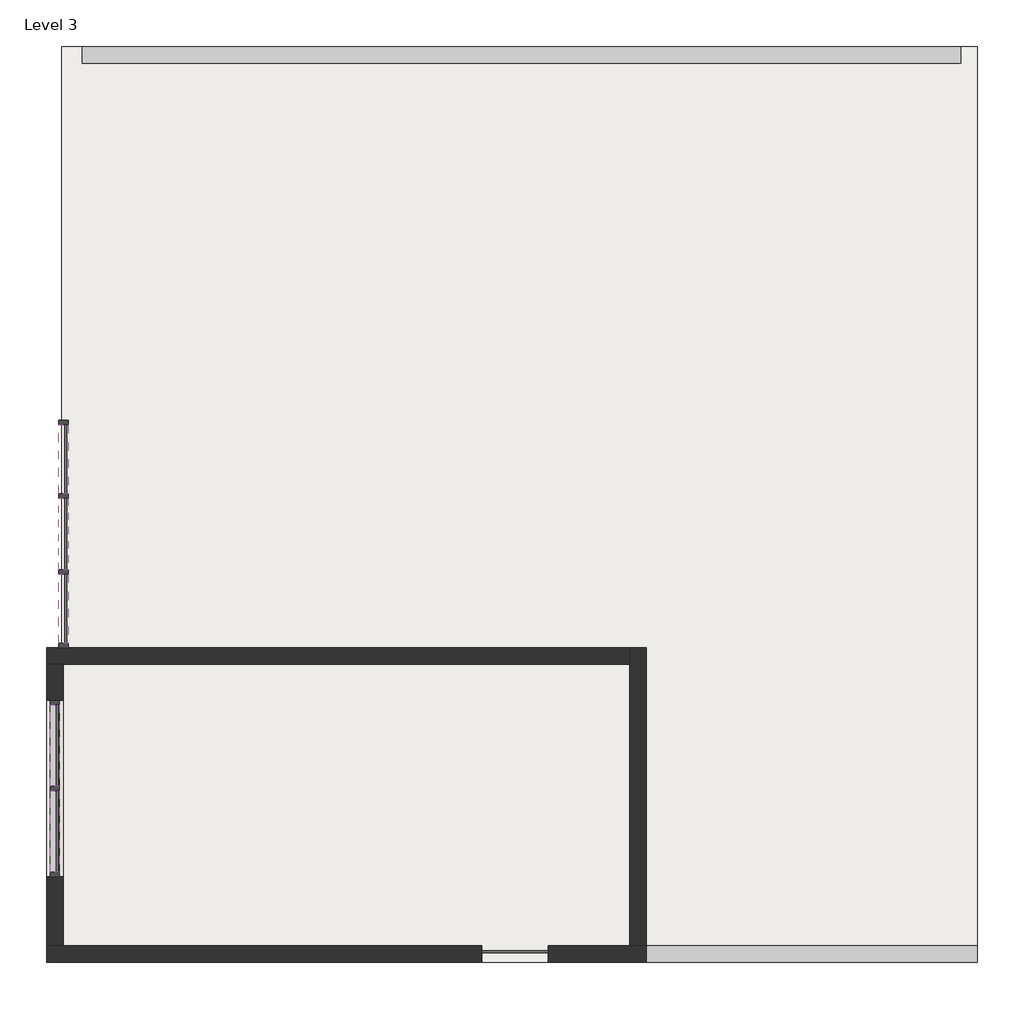
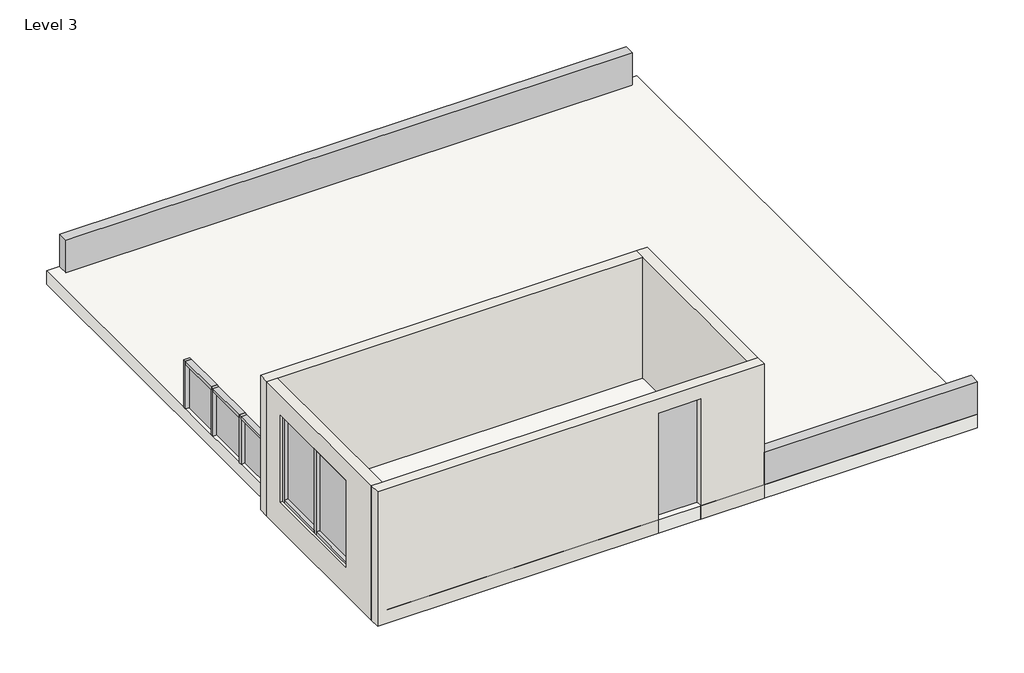
# One storey: 14 members, 7 plates, 4 walls, 2 proxies, 1 roof.
"""IFC4 building model written with IfcOpenShell, lengths in millimetres."""

from ifc_helpers import new_model, si_unit, frame, origin, place, context, project, spatial, polyline, outline, extrude, faceted_brep, transform, mapped, element, save
from components import generic_models_7_generic_models_7_f087c847, generic_models_9_generic_models_9_ac56366f, member_ade69111, member_05cf8435, member_3f9fbe84, member_9c6a9240, member_e6b9f524, member_bbdb212f, member_37619358, system_panel_glazed_77e7111d, system_panel_glazed_c8b910d9, system_panel_glazed_8012c4e8, system_panel_glazed_450ffc3c, system_panel_glazed_9aa1dd94

model = new_model("IFC4")

# Units and contexts
model_context = context("Model", 3, world=origin())
ifc_project = project(units=[si_unit("LENGTHUNIT", "METRE", prefix="MILLI")], contexts=[model_context])

# Site, building, storey
site = spatial("IfcSite", under=ifc_project)
building = spatial("IfcBuilding", under=site)
storey = spatial("IfcBuildingStorey", under=building, Name="Level 3", Elevation=6096.0)

# Proxies
placement = place(None, origin())
generic_models_7_generic_models_7_shape = generic_models_7_generic_models_7_f087c847(model_context)
element("IfcBuildingElementProxy", 1, Name="Generic Models 7 : Generic Models 7", ObjectType="Generic Models 7 : Generic Models 7", at=placement, inside=storey, context=model_context, shape_type="MappedRepresentation", body=[
    mapped(generic_models_7_generic_models_7_shape, transform((0.0, 0.0, 0.0), x_axis=(1.0, 0.0, 0.0), y_axis=(0.0, 1.0, 0.0), z_axis=(0.0, 0.0, 1.0))),
])
generic_models_9_generic_models_9_shape = generic_models_9_generic_models_9_ac56366f(model_context)
element("IfcBuildingElementProxy", 2, Name="Generic Models 9 : Generic Models 9", ObjectType="Generic Models 9 : Generic Models 9", at=placement, inside=storey, context=model_context, shape_type="MappedRepresentation", body=[
    mapped(generic_models_9_generic_models_9_shape, transform((0.0, 0.0, 0.0), x_axis=(1.0, 0.0, 0.0), y_axis=(0.0, 1.0, 0.0), z_axis=(0.0, 0.0, 1.0))),
])

# Members
member_shape = member_ade69111(model_context)
element("IfcMember", 3, ObjectType="Rectangular Mullion : 2.5\" x 5\" rectangular", at=placement, inside=storey, context=model_context, shape_type="MappedRepresentation", body=[
    mapped(member_shape, transform((-20241.3334471, -7434.170098, 6457.2827682), x_axis=(0.0, -1.0, 0.0), y_axis=(-1.0, 0.0, 0.0), z_axis=(0.0, 0.0, -1.0))),
])
element("IfcMember", 4, ObjectType="Rectangular Mullion : 2.5\" x 5\" rectangular", at=placement, inside=storey, context=model_context, shape_type="MappedRepresentation", body=[
    mapped(member_shape, transform((-20241.3334471, -8482.0613656, 6457.2827682), x_axis=(0.0, -1.0, 0.0), y_axis=(-1.0, 0.0, 0.0), z_axis=(0.0, 0.0, -1.0))),
])
member_2_shape = member_05cf8435(model_context)
element("IfcMember", 5, ObjectType="Rectangular Mullion : 2.5\" x 5\" rectangular", at=placement, inside=storey, context=model_context, shape_type="MappedRepresentation", body=[
    mapped(member_2_shape, transform((-20241.3334471, -8450.3113656, 7537.0329538), x_axis=(0.0, 0.0, 1.0), y_axis=(-1.0, 0.0, 0.0), z_axis=(0.0, -1.0, 0.0))),
])
member_3_shape = member_3f9fbe84(model_context)
element("IfcMember", 6, ObjectType="Rectangular Mullion : 2.5\" x 5\" rectangular", at=placement, inside=storey, context=model_context, shape_type="MappedRepresentation", body=[
    mapped(member_3_shape, transform((-20241.3334471, -7402.420098, 7537.0329538), x_axis=(0.0, 0.0, 1.0), y_axis=(-1.0, 0.0, 0.0), z_axis=(0.0, -1.0, 0.0))),
])
element("IfcMember", 7, ObjectType="Rectangular Mullion : 2.5\" x 5\" rectangular", at=placement, inside=storey, context=model_context, shape_type="MappedRepresentation", body=[
    mapped(member_3_shape, transform((-20241.3334471, -9466.4526331, 7537.0329538), x_axis=(0.0, 0.0, 1.0), y_axis=(-1.0, 0.0, 0.0), z_axis=(0.0, -1.0, 0.0))),
])
member_4_shape = member_9c6a9240(model_context)
element("IfcMember", 8, ObjectType="Rectangular Mullion : 2.5\" x 5\" rectangular", at=placement, inside=storey, context=model_context, shape_type="MappedRepresentation", body=[
    mapped(member_4_shape, transform((-20241.3334471, -6386.2788305, 7537.0329538), x_axis=(0.0, 1.0, 0.0), y_axis=(-1.0, 0.0, 0.0), z_axis=(0.0, 0.0, 1.0))),
])
element("IfcMember", 9, ObjectType="Rectangular Mullion : 2.5\" x 5\" rectangular", at=placement, inside=storey, context=model_context, shape_type="MappedRepresentation", body=[
    mapped(member_4_shape, transform((-20241.3334471, -9529.9526331, 6457.2827682), x_axis=(0.0, -1.0, 0.0), y_axis=(-1.0, 0.0, 0.0), z_axis=(0.0, 0.0, -1.0))),
])
member_5_shape = member_e6b9f524(model_context)
element("IfcMember", 10, ObjectType="Rectangular Mullion : 2.5\" x 5\" rectangular", at=placement, inside=storey, context=model_context, shape_type="MappedRepresentation", body=[
    mapped(member_5_shape, transform((-20360.0003587, -11441.3026331, 8684.6922049), x_axis=(0.0, 0.0, 1.0), y_axis=(-1.0, 0.0, 0.0), z_axis=(0.0, -1.0, 0.0))),
])
element("IfcMember", 11, ObjectType="Rectangular Mullion : 2.5\" x 5\" rectangular", at=placement, inside=storey, context=model_context, shape_type="MappedRepresentation", body=[
    mapped(member_5_shape, transform((-20360.0003587, -12628.7526331, 8684.6922049), x_axis=(0.0, 0.0, 1.0), y_axis=(-1.0, 0.0, 0.0), z_axis=(0.0, -1.0, 0.0))),
])
member_6_shape = member_bbdb212f(model_context)
element("IfcMember", 12, ObjectType="Rectangular Mullion : 2.5\" x 5\" rectangular", at=placement, inside=storey, context=model_context, shape_type="MappedRepresentation", body=[
    mapped(member_6_shape, transform((-20360.0003587, -11473.0526331, 6713.9016971), x_axis=(0.0, -1.0, 0.0), y_axis=(-1.0, 0.0, 0.0), z_axis=(0.0, 0.0, -1.0))),
])
element("IfcMember", 13, ObjectType="Rectangular Mullion : 2.5\" x 5\" rectangular", at=placement, inside=storey, context=model_context, shape_type="MappedRepresentation", body=[
    mapped(member_5_shape, transform((-20360.0003587, -11504.8026331, 6713.9016971), x_axis=(0.0, 0.0, -1.0), y_axis=(-1.0, 0.0, 0.0), z_axis=(0.0, 1.0, 0.0))),
])
element("IfcMember", 14, ObjectType="Rectangular Mullion : 2.5\" x 5\" rectangular", at=placement, inside=storey, context=model_context, shape_type="MappedRepresentation", body=[
    mapped(member_5_shape, transform((-20360.0003587, -10317.3526331, 6713.9016971), x_axis=(0.0, 0.0, -1.0), y_axis=(-1.0, 0.0, 0.0), z_axis=(0.0, 1.0, 0.0))),
])
member_7_shape = member_37619358(model_context)
element("IfcMember", 15, ObjectType="Rectangular Mullion : 2.5\" x 5\" rectangular", at=placement, inside=storey, context=model_context, shape_type="MappedRepresentation", body=[
    mapped(member_7_shape, transform((-20360.0003587, -10253.8526331, 8684.6922049), x_axis=(0.0, 1.0, 0.0), y_axis=(-1.0, 0.0, 0.0), z_axis=(0.0, 0.0, 1.0))),
])
element("IfcMember", 16, ObjectType="Rectangular Mullion : 2.5\" x 5\" rectangular", at=placement, inside=storey, context=model_context, shape_type="MappedRepresentation", body=[
    mapped(member_7_shape, transform((-20360.0003587, -12692.2526331, 6713.9016971), x_axis=(0.0, -1.0, 0.0), y_axis=(-1.0, 0.0, 0.0), z_axis=(0.0, 0.0, -1.0))),
])

# Plates
system_panel_glazed_shape = system_panel_glazed_77e7111d(model_context)
element("IfcPlate", 17, ObjectType="System Panel : Glazed", at=placement, inside=storey, context=model_context, shape_type="MappedRepresentation", body=[
    mapped(system_panel_glazed_shape, transform((-20241.3334471, -7958.1157318, 6457.2827682), x_axis=(0.0, -1.0, 0.0), y_axis=(1.0, 0.0, 0.0), z_axis=(0.0, 0.0, 1.0))),
])
system_panel_glazed_2_shape = system_panel_glazed_c8b910d9(model_context)
element("IfcPlate", 18, ObjectType="System Panel : Glazed", at=placement, inside=storey, context=model_context, shape_type="MappedRepresentation", body=[
    mapped(system_panel_glazed_2_shape, transform((-20241.3334471, -6926.0994643, 6457.2827682), x_axis=(0.0, -1.0, 0.0), y_axis=(1.0, 0.0, 0.0), z_axis=(0.0, 0.0, 1.0))),
])
element("IfcPlate", 19, ObjectType="System Panel : Glazed", at=placement, inside=storey, context=model_context, shape_type="MappedRepresentation", body=[
    mapped(system_panel_glazed_2_shape, transform((-20241.3334471, -8990.1319993, 6457.2827682), x_axis=(0.0, -1.0, 0.0), y_axis=(1.0, 0.0, 0.0), z_axis=(0.0, 0.0, 1.0))),
])
system_panel_glazed_3_shape = system_panel_glazed_8012c4e8(model_context)
element("IfcPlate", 20, ObjectType="System Panel : Glazed", at=placement, inside=storey, context=model_context, shape_type="MappedRepresentation", body=[
    mapped(system_panel_glazed_3_shape, transform((-20360.0003587, -10879.3276331, 6777.4016971), x_axis=(0.0, -1.0, 0.0), y_axis=(1.0, 0.0, 0.0), z_axis=(0.0, 0.0, 1.0))),
])
element("IfcPlate", 21, ObjectType="System Panel : Glazed", at=placement, inside=storey, context=model_context, shape_type="MappedRepresentation", body=[
    mapped(system_panel_glazed_3_shape, transform((-20360.0003587, -12066.7776331, 6777.4016971), x_axis=(0.0, -1.0, 0.0), y_axis=(1.0, 0.0, 0.0), z_axis=(0.0, 0.0, 1.0))),
])
system_panel_glazed_4_shape = system_panel_glazed_450ffc3c(model_context)
element("IfcPlate", 22, ObjectType="System Panel : Glazed", at=placement, inside=storey, context=model_context, shape_type="MappedRepresentation", body=[
    mapped(system_panel_glazed_4_shape, transform((-14003.6503587, -13759.0526331, 6096.0), x_axis=(1.0, 0.0, 0.0), y_axis=(0.0, 1.0, 0.0), z_axis=(0.0, 0.0, 1.0))),
])
system_panel_glazed_5_shape = system_panel_glazed_9aa1dd94(model_context)
element("IfcPlate", 23, ObjectType="System Panel : Glazed", at=placement, inside=storey, context=model_context, shape_type="MappedRepresentation", body=[
    mapped(system_panel_glazed_5_shape, transform((-14003.6503587, -13759.0526331, 6248.4), x_axis=(1.0, 0.0, 0.0), y_axis=(0.0, 1.0, 0.0), z_axis=(0.0, 0.0, 1.0))),
])

# Roof
element("IfcRoof", 24, ObjectType="Generic - 12\"", at=placement, inside=storey, context=model_context, shape_type="SweptSolid", body=[
    extrude(outline(polyline([(-20264.7503587, -1224.1526331), (-7615.5503587, -1224.1526331), (-7615.5503587, -13873.3526331), (-20264.7503587, -13873.3526331), (-20264.7503587, -1224.1526331)])), frame((0.0, 0.0, 6096.0), z_axis=(0.0, 0.0, 1.0), x_axis=(1.0, 0.0, 0.0)), (0.0, 0.0, 1.0), 304.8),
])

# Walls
element("IfcWall", 25, ObjectType="9\"", at=placement, inside=storey, context=model_context, shape_type="Brep", body=[
    faceted_brep([(-12187.5503587, -13873.3526331, 9144.0), (-20474.3003587, -13873.3526331, 9144.0), (-20474.3003587, -13873.3526331, 6096.0), (-14460.8503587, -13873.3526331, 6096.0), (-14460.8503587, -13873.3526331, 8818.9950276), (-13546.4503587, -13873.3526331, 8818.9950276), (-13546.4503587, -13873.3526331, 6096.0), (-12187.5503587, -13873.3526331, 6096.0), (-20474.3003587, -13644.7526331, 9144.0), (-20245.7003587, -13644.7526331, 9144.0), (-12416.1503587, -13644.7526331, 9144.0), (-12187.5503587, -13644.7526331, 9144.0), (-12187.5503587, -13644.7526331, 6096.0), (-12416.1503587, -13644.7526331, 6096.0), (-13546.4503587, -13644.7526331, 6096.0), (-13546.4503587, -13644.7526331, 8818.9950276), (-14460.8503587, -13644.7526331, 8818.9950276), (-14460.8503587, -13644.7526331, 6096.0), (-20245.7003587, -13644.7526331, 6096.0), (-20474.3003587, -13644.7526331, 6096.0)], [[[0, 1, 2, 3, 4, 5, 6, 7]], [[8, 9, 10, 11, 12, 13, 14, 15, 16, 17, 18, 19]], [[12, 7, 6, 14, 13]], [[2, 19, 18, 17, 3]], [[1, 0, 11, 10, 9, 8]], [[0, 7, 12, 11]], [[2, 1, 8, 19]], [[16, 4, 3, 17]], [[4, 16, 15, 5]], [[5, 15, 14, 6]]]),
])
element("IfcWall", 26, ObjectType="9\"", at=placement, inside=storey, context=model_context, shape_type="Brep", body=[
    faceted_brep([(-12187.5503587, -13644.7526331, 6096.0), (-12187.5503587, -9529.9526331, 6096.0), (-12187.5503587, -9529.9526331, 9144.0), (-12187.5503587, -13644.7526331, 9144.0), (-12416.1503587, -13644.7526331, 6096.0), (-12416.1503587, -13644.7526331, 9144.0), (-12416.1503587, -9758.5526331, 9144.0), (-12416.1503587, -9529.9526331, 9144.0), (-12416.1503587, -9529.9526331, 6096.0), (-12416.1503587, -9758.5526331, 6096.0)], [[[0, 1, 2, 3]], [[4, 5, 6, 7, 8, 9]], [[1, 0, 4, 9, 8]], [[3, 2, 7, 6, 5]], [[0, 3, 5, 4]], [[2, 1, 8, 7]]]),
])
element("IfcWall", 27, ObjectType="9\"", at=placement, inside=storey, context=model_context, shape_type="Brep", body=[
    faceted_brep([(-12416.1503587, -9529.9526331, 6096.0), (-20474.3003587, -9529.9526331, 6096.0), (-20474.3003587, -9529.9526331, 9144.0), (-12416.1503587, -9529.9526331, 9144.0), (-12416.1503587, -9758.5526331, 6096.0), (-12416.1503587, -9758.5526331, 9144.0), (-20245.7003587, -9758.5526331, 9144.0), (-20474.3003587, -9758.5526331, 9144.0), (-20474.3003587, -9758.5526331, 6096.0), (-20245.7003587, -9758.5526331, 6096.0)], [[[0, 1, 2, 3]], [[4, 5, 6, 7, 8, 9]], [[1, 0, 4, 9, 8]], [[3, 2, 7, 6, 5]], [[0, 3, 5, 4]], [[2, 1, 8, 7]]]),
])
element("IfcWall", 28, ObjectType="9\"", at=placement, inside=storey, context=model_context, shape_type="SweptSolid", body=[
    extrude(outline(polyline([(-9758.5526331, 6096.0), (-13644.7526331, 6096.0), (-13644.7526331, 9144.0), (-9758.5526331, 9144.0), (-9758.5526331, 6096.0)]), holes=[polyline([(-10253.8526331, 6713.9016971), (-10253.8526331, 8684.6922049), (-12692.2526331, 8684.6922049), (-12692.2526331, 6713.9016971), (-10253.8526331, 6713.9016971)])]), frame((-20474.3003587, 0.0, 0.0), z_axis=(1.0, 0.0, 0.0), x_axis=(0.0, 1.0, 0.0)), (0.0, 0.0, 1.0), 228.6),
])

save(model, "model.ifc")

# Revit data of these elements
# Type "Rectangular Mullion : 2.5\" x 5\" rectangular"
#   built-in parameter 1007304 = 0.416667 (stored number, unit not read)
#   built-in parameter 1007301 = 0.104167 (stored number, unit not read)
#   built-in parameter 1007300 = 0.104167 (stored number, unit not read)
# Type "System Panel : Glazed"
#   Construction Type Id = "GSP4R"
#   Analytic Construction = "1/8 in Pilkington single glazing"
#   Visual Light Transmittance = 0.9
#   Solar Heat Gain Coefficient = 0.86
#   Heat Transfer Coefficient (U) = 1.18115 BTU/(h·ft²·°F)
#   Define Thermal Properties by = 1
# Type "Generic - 12\""
#   Assembly Code = "B1020"
#   Layers, outside or top first: 1' - 0" no material (function 1)
# Type "9\""
#   Assembly Code = "B2010"
#   Layers, outside or top first: 0' - 9" no material (function 1)
# Element 1 (IfcBuildingElementProxy, "Generic Models 7 : Generic Models 7")
#   Phase Created = New Construction
# Element 2 (IfcBuildingElementProxy, "Generic Models 9 : Generic Models 9")
#   Phase Created = New Construction
# Elements 3, 4, 5, 6, 7, 8, 9, 10, 11, 12, 13, 14, 15, 16 (IfcMember, "Rectangular Mullion : 2.5\" x 5\" rectangular")
#   Phase Created = New Construction
#   Materials on its faces: "Aluminum"
# Elements 17, 18, 19, 20, 21, 22, 23 (IfcPlate, "System Panel : Glazed")
#   Phase Created = New Construction
#   Materials on its faces: "Glass"
# Element 24 (IfcRoof, "Generic - 12\"")
#   built-in parameter 1001705 = 21 (stored number, unit not read)
#   built-in parameter 1001710 = 33615
#   Phase Created = New Construction
#   Materials on its faces: "Default Roof"
# Elements 25, 26, 27, 28 (IfcWall, "9\"")
#   Top Offset = 0' - 0"
#   Base Offset = 0' - 0"
#   Unconnected Height = 10' - 0"
#   wall height = 10' - 0"
#   Phase Created = New Construction
#   Base Constraint = Level 3
#   Materials on its faces: "Default Wall"
# Materials
#   "Aluminum": class "Metal", colour RGB 247 247 247, transparency 0, Description = "Aluminum 6061", Cost = 0
#   "Glass": class "Glass", colour RGB 0 128 192, transparency 0.75, Description = "Soda Lime Glass", Cost = 0
#   "Default Roof": colour RGB 88 101 114, transparency 0, Cost = 0
#   "Default Wall": colour RGB 128 128 128, transparency 0, Cost = 0
